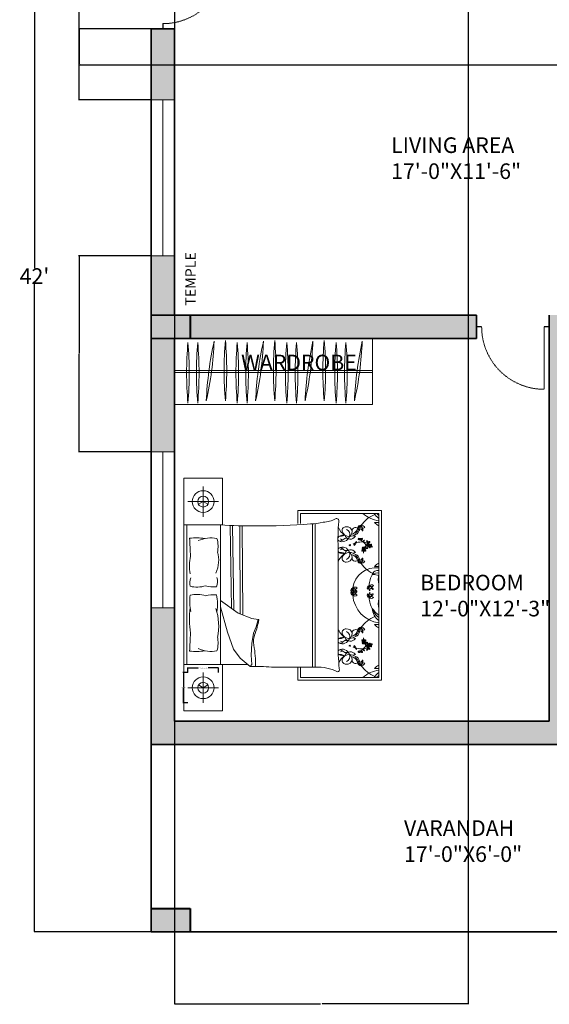
# Model space of a CAD drawing. Units: inches. Extents: x -10 to 455, y -513 to 57.
# Tile 1 of 4: x -10 to 193, y -513 to -134. Entities that reach past the tile are written whole.
import ezdxf

# ---------------------------------------------------------------- set-up
doc = ezdxf.new("R2010")
doc.units = ezdxf.units.IN
doc.header["$MEASUREMENT"] = 0
doc.linetypes.add('DASHED2', pattern=[0.375, 0.25, -0.125])
for name, color, linetype, lineweight in [('A-ANNO-DIMS', 2, 'Continuous', 18), ('A-ANNO-TEXT', 7, 'Continuous', 18), ('A-AREA-IDEN', 7, 'Continuous', 18), ('A-COLS', 7, 'Continuous', 40), ('A-COLS-PATT', 1, 'Continuous', 13), ('A-DOOR', 40, 'DASHED2', 18), ('A-DOOR-FRAM', 7, 'Continuous', 25), ('A-FLOR-CASE', 8, 'Continuous', 18), ('A-FURN', 8, 'Continuous', 13), ('A-GLAZ', 222, 'Continuous', 18), ('A-WALL', 7, 'Continuous', 35), ('A-WALL-PATT', 152, 'Continuous', 13)]:
    doc.layers.add(name, color=color, linetype=linetype, lineweight=lineweight)
doc.styles.get("Standard").update_dxf_attribs({"font": 'arial.ttf'})
doc.dimstyles.get("Standard").update_dxf_attribs({"dimtxt": 0.18, "dimasz": 0.18, "dimexe": 0.18, "dimexo": 0.0625, "dimgap": 0.09, "dimtad": 0, "dimtih": 1, "dimtoh": 1, "dimdec": 0, "dimzin": 0, "dimdsep": 46, "dimlunit": 3, "dimtxsty": 'Standard', "dimcen": 0.09, "dimadec": 0, "dimazin": 0, "dimtfac": 1, "dimtdec": 0, "dimtofl": 0, "dimtmove": 0, "dimatfit": 3, "dimfxl": 1, "dimtolj": 1, "dimtzin": 0, "dimarcsym": 0})

# ---------------------------------------------------------------- blocks, each defined once
blk = doc.blocks.new('*D2')
at = {"layer": 'A-ANNO-DIMS', "color": 0, "lineweight": -2, "transparency": 16777216}
for p, q in [((40.18, 19.15), (-4.74, 19.15)), ((-4.56, 18.97), (-4.56, -229.75)), ((-4.56, -484.67), (-4.56, -235.95)), ((40.18, -484.85), (-4.74, -484.85))]:
    blk.add_line(p, q, dxfattribs=at)
at = {"layer": 'A-ANNO-DIMS', "color": 0, "transparency": 16777216}
for points in [[(-4.59, 18.97), (-4.53, 18.97), (-4.56, 19.15)], [(-4.59, -484.67), (-4.53, -484.67), (-4.56, -484.85)]]:
    blk.add_solid(points, dxfattribs=at)
at = {"layer": 'Defpoints', "color": 0, "transparency": 16777216}
for p in [(40.25, 19.15), (-4.56, -484.85), (40.25, -484.85)]:
    blk.add_point(p, dxfattribs=at)
at = {"layer": 'A-ANNO-DIMS', "color": 0, "transparency": 16777216, "insert": (-4.56, -232.85), "char_height": 6, "attachment_point": 5}
blk.add_mtext("\\A1;42'", dxfattribs=at)
blk = doc.blocks.new('WIN-60IN')
for p, q in [((0, 9), (60, 9)), ((0, 0), (0, 9)), ((60, 9), (60, 0)), ((0, 4.5), (60, 4.5)), ((60, 0), (0, 0))]:
    blk.add_line(p, q)
blk = doc.blocks.new('DOOR-SINGLE-24IN')
for p, q in [((0, 28), (0, 26)), ((0, 26), (24, 26)), ((0, 0), (0, 2))]:
    blk.add_line(p, q)
blk.add_arc((0, 26), 24, 270, 0)
blk = doc.blocks.new('LAMP-BEDSIDE-SMALL')
for p, q in [((5.84, 0), (5.84, 11.68)), ((11.68, 5.84), (0, 5.84))]:
    blk.add_line(p, q)
for points in [[(5.84, 5.84), (4.03, 4.8)], [(5.84, 5.84), (7.65, 4.8)]]:
    blk.add_lwpolyline(points)
for radius in [4.17, 2.09]:
    blk.add_circle((5.84, 5.84), radius)
blk = doc.blocks.new('*D28')
at = {"layer": 'A-ANNO-DIMS', "color": 0, "lineweight": -2, "transparency": 16777216}
for p, q in [((54.41, -385.12), (54.41, -383.25)), ((54.59, -383.43), (58.38, -383.43)), ((65.92, -383.43), (62.13, -383.43)), ((66.1, -385.12), (66.1, -383.25))]:
    blk.add_line(p, q, dxfattribs=at)
at = {"layer": 'A-ANNO-DIMS', "color": 0, "transparency": 16777216}
for points in [[(54.59, -383.4), (54.59, -383.46), (54.41, -383.43)], [(65.92, -383.4), (65.92, -383.46), (66.1, -383.43)]]:
    blk.add_solid(points, dxfattribs=at)
at = {"layer": 'Defpoints', "color": 0, "transparency": 16777216}
for p in [(54.41, -383.43), (54.41, -385.18), (66.1, -385.18)]:
    blk.add_point(p, dxfattribs=at)
at = {"layer": 'A-ANNO-DIMS', "color": 0, "transparency": 16777216, "insert": (60.25, -383.43), "char_height": 0.18, "attachment_point": 5}
blk.add_mtext('\\A1;BEDSIDE LAMP 0\'-11 1/2" TYP.', dxfattribs=at)
blk = doc.blocks.new('*D29')
at = {"layer": 'A-ANNO-DIMS', "color": 0, "lineweight": -2, "transparency": 16777216}
for p, q in [((54.35, -385.18), (52.48, -385.18)), ((52.66, -385.36), (52.66, -390.84)), ((52.66, -396.68), (52.66, -391.2)), ((54.35, -396.86), (52.48, -396.86))]:
    blk.add_line(p, q, dxfattribs=at)
at = {"layer": 'A-ANNO-DIMS', "color": 0, "transparency": 16777216}
for points in [[(52.63, -385.36), (52.69, -385.36), (52.66, -385.18)], [(52.63, -396.68), (52.69, -396.68), (52.66, -396.86)]]:
    blk.add_solid(points, dxfattribs=at)
at = {"layer": 'Defpoints', "color": 0, "transparency": 16777216}
for p in [(54.41, -385.18), (52.66, -396.86), (54.41, -396.86)]:
    blk.add_point(p, dxfattribs=at)
at = {"layer": 'A-ANNO-DIMS', "color": 0, "transparency": 16777216, "insert": (52.66, -391.02), "char_height": 0.18, "attachment_point": 5}
blk.add_mtext('\\A1;0\'-11 1/2" TYP.', dxfattribs=at)
blk = doc.blocks.new('*D35')
at = {"layer": 'A-ANNO-DIMS', "color": 0, "lineweight": -2, "transparency": 16777216}
for p, q in [((40.18, -137.85), (12.42, -137.85)), ((12.6, -138.03), (12.6, -151.3)), ((12.6, -164.93), (12.6, -151.67)), ((40.18, -165.11), (12.42, -165.11))]:
    blk.add_line(p, q, dxfattribs=at)
at = {"layer": 'A-ANNO-DIMS', "color": 0, "transparency": 16777216}
for points in [[(12.57, -138.03), (12.63, -138.03), (12.6, -137.85)], [(12.57, -164.93), (12.63, -164.93), (12.6, -165.11)]]:
    blk.add_solid(points, dxfattribs=at)
at = {"layer": 'Defpoints', "color": 0, "transparency": 16777216}
for p in [(40.25, -137.85), (12.6, -165.11), (40.25, -165.11)]:
    blk.add_point(p, dxfattribs=at)
at = {"layer": 'A-ANNO-DIMS', "color": 0, "transparency": 16777216, "insert": (12.6, -151.48), "char_height": 0.18, "attachment_point": 5}
blk.add_mtext('\\A1;2\'-3 1/2"', dxfattribs=at)
blk = doc.blocks.new('*D36')
at = {"layer": 'A-ANNO-DIMS', "color": 0, "lineweight": -2, "transparency": 16777216}
for p, q in [((40.18, -225.11), (12.42, -225.11)), ((12.6, -225.29), (12.6, -262.55)), ((12.6, -300.17), (12.6, -262.91)), ((40.18, -300.35), (12.42, -300.35))]:
    blk.add_line(p, q, dxfattribs=at)
at = {"layer": 'A-ANNO-DIMS', "color": 0, "transparency": 16777216}
for points in [[(12.57, -225.29), (12.63, -225.29), (12.6, -225.11)], [(12.57, -300.17), (12.63, -300.17), (12.6, -300.35)]]:
    blk.add_solid(points, dxfattribs=at)
at = {"layer": 'Defpoints', "color": 0, "transparency": 16777216}
for p in [(40.25, -225.11), (12.6, -300.35), (40.25, -300.35)]:
    blk.add_point(p, dxfattribs=at)
at = {"layer": 'A-ANNO-DIMS', "color": 0, "transparency": 16777216, "insert": (12.6, -262.73), "char_height": 0.18, "attachment_point": 5}
blk.add_mtext('\\A1;6\'-3"', dxfattribs=at)
blk = doc.blocks.new('*D43')
at = {"layer": 'A-ANNO-DIMS', "color": 0, "lineweight": -2, "transparency": 16777216}
for p, q in [((253.18, -109.85), (12.42, -109.85)), ((12.6, -110.03), (12.6, -130.67)), ((12.6, -151.67), (12.6, -131.03)), ((253.18, -151.85), (12.42, -151.85))]:
    blk.add_line(p, q, dxfattribs=at)
at = {"layer": 'A-ANNO-DIMS', "color": 0, "transparency": 16777216}
for points in [[(12.57, -110.03), (12.63, -110.03), (12.6, -109.85)], [(12.57, -151.67), (12.63, -151.67), (12.6, -151.85)]]:
    blk.add_solid(points, dxfattribs=at)
at = {"layer": 'Defpoints', "color": 0, "transparency": 16777216}
for p in [(253.25, -109.85), (12.6, -151.85), (253.25, -151.85)]:
    blk.add_point(p, dxfattribs=at)
at = {"layer": 'A-ANNO-DIMS', "color": 0, "transparency": 16777216, "insert": (12.6, -130.85), "char_height": 0.18, "attachment_point": 5}
blk.add_mtext('\\A1;3\'-6"', dxfattribs=at)
blk = doc.blocks.new('*D44')
at = {"layer": 'A-ANNO-DIMS', "color": 0, "lineweight": -2, "transparency": 16777216}
for p, q in [((49.25, 10.09), (49.25, -512.68)), ((162.09, 10.09), (162.09, -512.68)), ((49.43, -512.5), (105.34, -512.5)), ((161.91, -512.5), (106, -512.5))]:
    blk.add_line(p, q, dxfattribs=at)
at = {"layer": 'A-ANNO-DIMS', "color": 0, "transparency": 16777216}
for points in [[(49.43, -512.47), (49.43, -512.53), (49.25, -512.5)], [(161.91, -512.47), (161.91, -512.53), (162.09, -512.5)]]:
    blk.add_solid(points, dxfattribs=at)
at = {"layer": 'Defpoints', "color": 0, "transparency": 16777216}
for p in [(49.25, 10.15), (162.09, 10.15), (162.09, -512.5)]:
    blk.add_point(p, dxfattribs=at)
at = {"layer": 'A-ANNO-DIMS', "color": 0, "transparency": 16777216, "insert": (105.67, -512.5), "char_height": 0.18, "attachment_point": 5}
blk.add_mtext('\\A1;9\'-5"', dxfattribs=at)

msp = doc.modelspace()

# ---------------------------------------------------------------- hatches: boundary and pattern name
at = {"layer": 'A-COLS-PATT'}
h = msp.add_hatch(color=256, dxfattribs=at)
h.dxf.hatch_style = 1
h.paths.add_polyline_path([(55.25, 19.15), (40.25, 19.15), (40.25, 10.15), (55.25, 10.15)])
h.paths.add_polyline_path([(262.25, 19.15), (253.25, 19.15), (253.25, 4.15), (262.25, 4.15)])
h.paths.add_polyline_path([(427.25, 19.15), (418.25, 19.15), (418.25, 4.15), (427.25, 4.15)])
h.paths.add_polyline_path([(427.25, -247.85), (418.25, -247.85), (418.25, -262.85), (427.25, -262.85)])
h.paths.add_polyline_path([(268.25, -247.85), (253.25, -247.85), (253.25, -256.85), (268.25, -256.85)])
h.paths.add_polyline_path([(55.25, -247.85), (40.25, -247.85), (40.25, -256.85), (55.25, -256.85)])
h.paths.add_polyline_path([(55.25, -475.85), (49.25, -475.85), (40.25, -475.85), (40.25, -484.85), (55.25, -484.85)])
h.paths.add_polyline_path([(268.25, -475.85), (253.25, -475.85), (253.25, -484.85), (268.25, -484.85)])
h.paths.add_polyline_path([(427.25, -469.85), (418.25, -469.85), (418.25, -484.85), (427.25, -484.85)])
h.paths.add_polyline_path([(55.25, -100.85), (40.25, -100.85), (40.25, -109.85), (55.25, -109.85)])
at = {"layer": 'A-WALL-PATT'}
h = msp.add_hatch(color=256, dxfattribs=at)
h.dxf.hatch_style = 1
h.paths.add_polyline_path([(418.25, -151.85), (268.25, -151.85), (268.25, -160.85), (418.25, -160.85)])
h.paths.add_polyline_path([(165.25, -100.85), (55.25, -100.85), (55.25, -109.85), (165.25, -109.85), (165.25, -105.35)])
h.paths.add_polyline_path([(49.25, -75.35), (40.25, -75.35), (40.25, -100.85), (49.25, -100.85)])
h.paths.add_polyline_path([(49.25, 10.15), (40.25, 10.15), (40.25, -15.35), (49.25, -15.35)])
h.paths.add_polyline_path([(86.75, 19.15), (55.25, 19.15), (55.25, 10.15), (86.75, 10.15)])
h.paths.add_polyline_path([(213.5, 19.15), (146.75, 19.15), (146.75, 10.15), (193.25, 10.15), (193.25, -28.04), (197.75, -28.04), (197.75, 10.15), (213.5, 10.15)])
h.paths.add_polyline_path([(262.25, 4.15), (253.25, 4.15), (253.25, -69.35), (197.75, -69.35), (197.75, -60), (193.25, -60), (193.25, -109.85), (197.75, -109.85), (197.75, -73.85), (253.25, -73.85), (253.25, -109.85), (262.25, -109.85)])
h.paths.add_polyline_path([(310.25, 19.15), (262.25, 19.15), (262.25, 10.15), (310.25, 10.15)])
h.paths.add_polyline_path([(253.25, 19.15), (237.5, 19.15), (237.5, 10.15), (253.25, 10.15)])
h.paths.add_polyline_path([(418.25, 19.15), (370.25, 19.15), (370.25, 10.15), (418.25, 10.15)])
h.paths.add_polyline_path([(427.25, 4.15), (418.25, 4.15), (418.25, -42.17), (427.25, -42.17)])
h.paths.add_polyline_path([(427.25, -102.17), (418.25, -102.17), (418.25, -145.85), (427.25, -145.85)])
h.paths.add_polyline_path([(427.25, -160.85), (418.25, -160.85), (418.25, -247.85), (427.25, -247.85)])
h.paths.add_polyline_path([(418.25, -247.85), (365.75, -247.85), (365.75, -256.85), (418.25, -256.85)], flags=17)
h.paths.add_polyline_path([(297.25, -247.85), (268.25, -247.85), (268.25, -256.85), (297.25, -256.85), (297.25, -252.35)], flags=17)
h.paths.add_polyline_path([(427.25, -299.44), (418.25, -299.44), (418.25, -319.85), (370.25, -319.85), (370.25, -284.85), (368, -284.85), (365.75, -284.85), (365.75, -319.85), (329.75, -319.85), (329.75, -247.85), (325.25, -247.85), (325.25, -319.85), (257.75, -319.85), (257.75, -256.85), (253.25, -256.85), (253.25, -324.35), (262.25, -324.35), (418.25, -324.35), (418.25, -363.39), (427.25, -363.39)])
h.paths.add_polyline_path([(262.25, -352.35), (257.75, -352.35), (253.25, -352.35), (253.25, -447.85), (257.75, -447.85), (262.25, -447.85)])
h.paths.add_polyline_path([(305.75, -475.85), (268.25, -475.85), (268.25, -484.85), (305.75, -484.85)])
h.paths.add_polyline_path([(418.25, -475.85), (365.75, -475.85), (365.75, -484.85), (418.25, -484.85)])
h.paths.add_polyline_path([(427.25, -423.39), (418.25, -423.39), (418.25, -469.85), (427.25, -469.85)])
h.paths.add_polyline_path([(202.25, -247.85), (193.25, -247.85), (193.25, -403.85), (49.25, -403.85), (49.25, -360.35), (40.25, -360.35), (40.25, -412.85), (202.25, -412.85)])
h.paths.add_polyline_path([(165.25, -247.85), (55.25, -247.85), (55.25, -256.85), (165.25, -256.85), (165.25, -252.35)], flags=17)
h.paths.add_polyline_path([(49.25, -225.11), (40.25, -225.11), (40.25, -247.85), (49.25, -247.85)])
h.paths.add_polyline_path([(49.25, -256.85), (40.25, -256.85), (40.25, -300.35), (49.25, -300.35)], flags=17)
h.paths.add_polyline_path([(49.25, -137.85), (44.75, -137.85), (40.25, -137.85), (40.25, -165.11), (49.25, -165.11)])

# ---------------------------------------------------------------- linework, layer by layer
at = {"layer": 'A-COLS'}
for p, q in [((55.25, -247.85), (55.25, -256.85)), ((40.25, -475.85), (49.25, -475.85)), ((49.25, -475.85), (55.25, -475.85)), ((55.25, -475.85), (55.25, -484.85))]:
    msp.add_line(p, q, dxfattribs=at)
at = {"layer": 'A-DOOR-FRAM'}
for p, q in [((44.75, -135.85), (44.75, -137.85)), ((167.25, -252.35), (165.25, -252.35)), ((193.25, -252.35), (191.25, -252.35))]:
    msp.add_line(p, q, dxfattribs=at)
at = {"layer": 'A-FLOR-CASE'}
for p, q in [((125.31, -256.85), (49.25, -256.85)), ((49.25, -256.85), (49.25, -282.2)), ((125.31, -256.85), (125.31, -282.2)), ((125.31, -269.1), (49.25, -269.1)), ((125.31, -269.95), (49.25, -269.95)), ((125.31, -282.2), (49.25, -282.2))]:
    msp.add_line(p, q, dxfattribs=at)
for centre, start, end in [((187.3, -270.03), 175.0028, 184.9972), ((-78.5, -270.03), 355.0028, 4.9972), ((191.06, -270.03), 175.0028, 184.9972), ((-74.74, -270.03), 355.0028, 4.9972), ((-68.8, -251.99), 347.508, 357.5023), ((194.73, -286.66), 167.508, 177.5023), ((201.69, -269.22), 175.0028, 184.9972), ((-64.11, -269.22), 355.0028, 4.9972), ((206.26, -270.03), 175.0028, 184.9972), ((-59.54, -270.03), 355.0028, 4.9972), ((210.01, -270.03), 175.0028, 184.9972), ((-55.79, -270.03), 355.0028, 4.9972), ((-49.85, -251.99), 347.508, 357.5023), ((213.68, -286.66), 167.508, 177.5023), ((220.64, -269.22), 175.0028, 184.9972), ((-45.16, -269.22), 355.0028, 4.9972), ((225.28, -270.03), 175.0028, 184.9972), ((-40.52, -270.03), 355.0028, 4.9972), ((229.03, -270.03), 175.0028, 184.9972), ((-36.77, -270.03), 355.0028, 4.9972), ((232.7, -286.66), 167.508, 177.5023), ((-30.83, -251.99), 347.508, 357.5023), ((239.66, -269.22), 175.0028, 184.9972), ((-26.14, -269.22), 355.0028, 4.9972), ((244.23, -270.03), 175.0028, 184.9972), ((-21.57, -270.03), 355.0028, 4.9972), ((247.98, -270.03), 175.0028, 184.9972), ((-17.82, -270.03), 355.0028, 4.9972), ((251.65, -286.66), 167.508, 177.5023), ((-11.88, -251.99), 347.508, 357.5023)]:
    msp.add_arc(centre, 133.41, start, end, dxfattribs=at)
at = {"layer": 'A-FURN'}
for p, q in [((52.81, -399.96), (52.81, -310.56)), ((96.63, -327.95), (96.63, -322.99)), ((96.63, -322.99), (128.83, -322.99)), ((97.66, -324.02), (97.66, -327.96)), ((127.79, -324.02), (97.66, -324.02)), ((127.79, -387.12), (127.79, -324.02)), ((128.83, -322.99), (128.83, -388.16)), ((53.95, -328.44), (53.95, -382.08)), ((66.93, -382.08), (66.93, -328.44)), ((70.65, -328.68), (71.09, -360.51)), ((71.56, -328.72), (72.02, -361.18)), ((74.38, -328.76), (74.51, -362.71)), ((75.3, -328.76), (75.44, -363.06)), ((102.2, -328.04), (102.2, -383.11)), ((103.32, -327.95), (103.32, -383.11)), ((118.73, -332.83), (117.72, -332.64)), ((112.1, -337.11), (112.1, -373.41)), ((118.73, -339.08), (117.72, -339.28)), ((66.93, -357.52), (73.75, -362.42)), ((69.59, -369.66), (66.93, -359.92)), ((73.75, -362.42), (79, -364.41)), ((79, -364.41), (81.35, -364.78)), ((81.35, -364.78), (80.63, -367.67)), ((71.94, -376.18), (69.59, -369.66)), ((79.54, -370.03), (79, -374.01)), ((80.63, -367.67), (79.54, -370.03)), ((79, -374.01), (78.64, -378.54)), ((118.73, -372.07), (117.72, -371.87)), ((74.47, -379.62), (71.94, -376.18)), ((118.73, -378.32), (117.72, -378.51)), ((52.81, -382.08), (77.34, -382.08)), ((78.27, -382.88), (74.47, -379.62)), ((78.64, -378.54), (79, -382.16)), ((79, -382.16), (78.27, -382.88)), ((96.63, -388.16), (96.63, -383.1)), ((97.66, -383.11), (97.66, -387.12)), ((128.83, -388.16), (96.63, -388.16)), ((97.66, -387.12), (127.79, -387.12))]:
    msp.add_line(p, q, dxfattribs=at)
for points in [[(52.81, -328.44), (67.7, -328.44), (67.7, -310.56), (52.81, -310.56)], [(67.7, -382.08), (67.7, -399.96), (52.81, -399.96)]]:
    msp.add_lwpolyline(points, dxfattribs=at)
for points in [[(101.5, -328.06, 0.056112), (106.42, -327.41, 0.095341), (111.15, -326.16)], [(55.03, -333.58, -0.074897), (60.87, -333.69, 0.472817)], [(61.2, -351.86, -0.14099), (55.24, -352.04, -0.235245)], [(61.2, -355.68, 0.14099), (55.24, -355.5, 0.235245)], [(55.03, -376.95, 0.074897), (60.87, -376.84, -0.472817)], [(86.46, -383.07, 0.001242), (103.42, -383.11, -0.127202), (111.88, -384.9)]]:
    msp.add_lwpolyline(points, format="xyb", dxfattribs=at)
for centre in [(124.37, -336.51), (121.97, -338), (121.97, -373.15), (124.37, -374.64)]:
    msp.add_circle(centre, 0.228, dxfattribs=at)
for centre, radius, start, end in [((130.52, -335.3), 11.67, 111.4092, 145.6135), ((129.37, -315.33), 11.67, 228.1144, 262.255), ((130.93, -321.19), 5.69, 209.8884, 236.5383), ((131.99, -319.14), 7.09, 223.5186, 233.6964), ((77.86, -168.19), 160.63, 266.1, 270.9282), ((83.7, -119.29), 209.53, 269.1145, 274.8735), ((111.61, -326.83), 0.815, 336.5219, 123.8264), ((199.04, -334.38), 86.99, 175.2402, 181.8035), ((115.15, -330.66), 1.51, 88.9462, 185.5144), ((115.36, -331.28), 2.14, 7.1143, 95.0551), ((120.66, -329.65), 0.968, 76.272, 177.0484), ((119.19, -327.67), 1.99, 284.7031, 328.6173), ((121.97, -330.21), 1.85, 125.7657, 194.5347), ((112.92, -326.94), 8.17, 332.8176, 347.4827), ((121.16, -329.98), 1.29, 20.9613, 102.2885), ((121.86, -328.68), 0.975, 181.7131, 301.5367), ((118.67, -330.65), 2.95, 2.0648, 41.1598), ((120.44, -329.56), 0.955, 316.2238, 62.3173), ((129.61, -324.38), 4.75, 221.0454, 247.4453), ((127.06, -311.37), 16.15, 266.3481, 272.5919), ((113.09, -333.79), 1.08, 127.675, 162.5814), ((112.76, -329.2), 3.7, 259.249, 301.1782), ((118.39, -326.72), 6.77, 203.6453, 236.3329), ((114.37, -335.79), 3.45, 85.2696, 124.215), ((116.26, -330.2), 2.69, 193.079, 274.7067), ((116.8, -331.73), 2.22, 196.8663, 330.0915), ((114.55, -332.12), 2.07, 338.5779, 68.4181), ((114.37, -335.79), 3.45, 53.6555, 57.2989), ((114.89, -330.91), 2.6, 305.9599, 357.6409), ((116.19, -328.09), 4.8, 273.4924, 303.7117), ((115.85, -328.13), 4.22, 288.2955, 328.7386), ((118.8, -330.79), 1.34, 19.1312, 189.736), ((118.4, -330.47), 1.68, 285.6955, 4.031), ((120.63, -332.27), 1.78, 128.4175, 173.8338), ((120.26, -330.51), 0.822, 126.7319, 206.0245), ((120.99, -330.12), 0.0761, 20.2667, 316.2271), ((121.4, -330.54), 0.0704, 52.0591, 168.5166), ((121.47, -330.55), 0.145, 168.5166, 2.0648), ((-795.72, -382.85), 852.18, 2.85022, 3.31479), ((63.22, -344.97), 11.52, 78.2417, 114.8684), ((53.99, -336.77), 11.98, 348.9631, 14.8961), ((113.09, -333.79), 1.08, 196.6343, 225.5483), ((113.72, -332.07), 2.85, 240.8249, 340.7178), ((112.87, -333.33), 1.34, 246.1646, 318.4347), ((114.24, -331.64), 2.57, 240.0851, 262.564), ((115.25, -335.44), 1.83, 74.8529, 138.4347), ((115.87, -333.13), 0.555, 254.8529, 12.6959), ((116.61, -336.19), 0.28, 169.5864, 349.5616), ((116.71, -336.21), 0.172, 349.5616, 167.2949), ((121.21, -342.41), 7.4, 110.1059, 116.9968), ((117.38, -335.22), 1.41, 308.4388, 328.836), ((118.73, -336.31), 0.469, 129.5056, 182.6421), ((117.13, -334.07), 2.52, 296.5064, 305.3102), ((117.11, -335.37), 1.44, 336.3901, 344.4871), ((118.68, -335.74), 0.182, 83.9457, 185.6216), ((117.95, -335.57), 0.749, 328.836, 0.8141), ((118.34, -335.79), 0.429, 306.5232, 32.4668), ((118.85, -335.45), 0.182, 112.5583, 214.2343), ((118.73, -335.13), 0.429, 265.7131, 351.6568), ((118.35, -334.89), 0.749, 297.3659, 329.344), ((117.79, -334.25), 1.44, 313.6929, 321.7899), ((119.38, -335.23), 0.469, 115.5379, 168.6744), ((117.78, -334.55), 1.41, 329.344, 349.7412), ((121.21, -342.41), 7.4, 86.1723, 106.4158), ((116.65, -334.88), 2.52, 352.8698, 1.6736), ((119.99, -333.97), 0.176, 125.0752, 284.7644), ((120.26, -333.9), 0.38, 127.3642, 168.4363), ((119.97, -333.59), 0.547, 277.4968, 341.2737), ((120.4, -333.85), 0.217, 88.1325, 178.8919), ((120.84, -334.08), 0.471, 136.3462, 189.6513), ((120.57, -334.13), 0.196, 189.6513, 312.3208), ((120.62, -333.58), 0.228, 183.2768, 356.7232), ((121.33, -333.99), 0.745, 164.2829, 186.9148), ((120.45, -334), 0.373, 312.3208, 40.2111), ((121.24, -333.58), 0.529, 201.6382, 274.947), ((120.54, -334.3), 0.691, 42.3896, 66.5724), ((127.51, -328.83), 8.49, 217.9541, 226.8459), ((121.04, -333.89), 0.376, 10.9597, 52.2379), ((121.27, -333.93), 0.175, 274.947, 37.5263), ((121.86, -334.92), 0.182, 112.5583, 214.2343), ((121.74, -334.59), 0.429, 265.7131, 351.6568), ((121.36, -334.36), 0.749, 297.3659, 329.344), ((121.4, -338.72), 3.71, 60.7959, 85.244), ((113.49, -344.07), 12.21, 37.8256, 47.7588), ((120.79, -333.71), 1.44, 313.6929, 321.7899), ((122.38, -334.69), 0.469, 115.5379, 168.6744), ((120.79, -334.02), 1.41, 329.344, 349.7412), ((119.66, -334.34), 2.52, 352.8698, 1.6736), ((126.33, -339.1), 4.45, 130.182, 149.456), ((123.21, -334.85), 0.254, 33.0979, 123.1364), ((117.61, -338.44), 6.65, 31.1156, 34.8118), ((122.84, -335.29), 0.688, 2.3172, 70.5201), ((123.88, -336.57), 0.734, 139.3812, 199.9959), ((122.51, -336.03), 1.04, 310.9365, 22.7695), ((122.98, -336.09), 0.754, 285.6484, 332.2957), ((123.41, -335.46), 0.199, 135.7354, 318.1297), ((123.08, -335.14), 0.263, 315.7354, 31.1156), ((122.86, -335.69), 0.611, 319.3812, 5.5456), ((123.56, -335.46), 0.199, 68.2452, 250.6395), ((123.1, -335.21), 0.593, 352.6008, 57.1845), ((125.22, -339.19), 3.97, 111.7087, 116.2181), ((121.4, -338.72), 3.71, 47.5083, 55.9967), ((123.66, -335.08), 0.593, 252.8042, 349.6943), ((123.1, -336.14), 0.631, 331.1838, 51.6792), ((123.73, -335.03), 0.263, 248.2452, 323.6254), ((124.02, -336.82), 0.38, 93.635, 168.4363), ((123.49, -334.87), 0.688, 291.7087, 3.0299), ((123.97, -336.22), 0.223, 138.2946, 276.2474), ((123.72, -336.52), 0.547, 277.4968, 341.2737), ((124.05, -336.26), 0.31, 358.5719, 143.8954), ((118.58, -331.24), 6.65, 323.6254, 327.3216), ((124.15, -336.77), 0.217, 88.1325, 178.8919), ((124.23, -336.01), 0.313, 208.8493, 269.9355), ((123.97, -336.09), 0.358, 274.2123, 318.1587), ((124.59, -337.01), 0.471, 136.3462, 189.6513), ((124.04, -335.04), 0.254, 325.6077, 55.6462), ((125.08, -336.92), 0.745, 164.2829, 186.9148), ((125.06, -336.45), 0.718, 121.9501, 165.2442), ((124.2, -336.92), 0.373, 312.3208, 40.2111), ((124.99, -336.5), 0.529, 201.6382, 274.947), ((124.56, -336.17), 0.151, 262.868, 7.094), ((124.29, -337.22), 0.691, 42.3896, 66.5724), ((124.54, -336.05), 0.449, 278.5614, 22.5914), ((124.79, -336.82), 0.376, 10.9597, 118.7804), ((124.8, -336.03), 0.226, 44.3732, 121.9501), ((70.68, -344.19), 15.72, 166.3427, 191.1841), ((54.87, -341.94), 11.38, 333.8761, 16.1746), ((113.09, -338.13), 1.08, 134.4517, 156.7144), ((113.09, -338.13), 1.08, 203.2856, 232.325), ((112.76, -342.71), 3.7, 58.8218, 100.2867), ((118.39, -345.19), 6.77, 123.6671, 158.5059), ((113.72, -339.84), 2.85, 19.2822, 119.1751), ((112.87, -338.58), 1.34, 41.5653, 113.8354), ((114.37, -336.13), 3.45, 235.785, 274.7304), ((114.24, -340.27), 2.57, 97.436, 119.9149), ((116.26, -341.72), 2.69, 85.2933, 166.921), ((115.25, -336.48), 1.83, 221.5653, 285.1471), ((116.8, -340.19), 2.22, 29.9085, 163.1337), ((114.55, -339.79), 2.07, 291.5819, 21.4221), ((115.87, -338.78), 0.555, 347.3041, 105.1471), ((114.37, -336.13), 3.45, 302.7011, 306.3445), ((114.89, -341.01), 2.6, 2.3591, 54.0401), ((116.19, -343.83), 4.8, 56.2883, 86.5076), ((115.85, -343.79), 4.22, 31.2614, 71.7045), ((120.63, -339.64), 1.78, 186.1662, 231.5825), ((118.4, -341.45), 1.68, 355.969, 74.3045), ((121.35, -338.38), 0.176, 125.0752, 284.7644), ((121.62, -338.31), 0.38, 93.635, 168.4363), ((121.63, -336.26), 1.04, 253.6301, 325.4631), ((121.92, -337.7), 0.734, 82.0748, 142.6895), ((121.84, -336.69), 0.754, 228.342, 274.9894), ((121.57, -337.71), 0.223, 138.2946, 276.2474), ((121.32, -338.01), 0.547, 277.4968, 341.2737), ((121.65, -337.75), 0.31, 358.5719, 143.8954), ((121.75, -338.26), 0.217, 88.1325, 178.8919), ((121.83, -337.5), 0.313, 208.8493, 269.9355), ((121.57, -337.58), 0.358, 274.2123, 318.1587), ((122.19, -338.49), 0.471, 136.3462, 189.6513), ((121.92, -338.54), 0.196, 189.6513, 312.3208), ((126.33, -339.1), 4.45, 175.2415, 182.8929), ((121.86, -336.81), 0.631, 273.8774, 357.1501), ((122.68, -338.4), 0.745, 164.2829, 186.9148), ((122.66, -337.94), 0.718, 121.9501, 165.2442), ((122.11, -336.36), 0.611, 262.0748, 308.2393), ((121.8, -338.41), 0.373, 312.3208, 40.2111), ((122.59, -337.99), 0.529, 201.6382, 274.947), ((122.16, -337.66), 0.151, 262.868, 7.094), ((121.89, -338.71), 0.691, 42.3896, 66.5724), ((122.14, -337.53), 0.449, 278.5614, 22.5914), ((122.39, -338.31), 0.376, 10.9597, 118.7804), ((126.33, -339.1), 4.45, 156.1523, 156.9499), ((122.4, -337.52), 0.226, 44.3732, 121.9501), ((123.09, -336.99), 0.631, 181.4625, 249.4747), ((122.99, -336.49), 0.611, 215.1128, 261.2773), ((123.47, -336.52), 1.04, 197.889, 269.722), ((122.62, -338.34), 0.175, 274.947, 37.5263), ((123.15, -336.88), 0.754, 248.3627, 295.0101), ((122.78, -337.82), 0.734, 20.6625, 81.2773), ((123.75, -336.89), 0.176, 125.0752, 284.7644), ((124.32, -337.05), 0.196, 189.6513, 312.3208), ((125.02, -336.85), 0.175, 274.947, 37.5263), ((115.15, -341.25), 1.51, 174.4856, 271.0538), ((115.36, -340.63), 2.14, 264.9449, 352.8857), ((118.8, -341.13), 1.34, 170.264, 340.8688), ((120.26, -341.4), 0.822, 153.9755, 233.2681), ((120.66, -342.26), 0.968, 182.9516, 283.728), ((119.19, -344.24), 1.99, 31.3827, 75.2969), ((121.97, -341.7), 1.85, 165.4653, 234.2343), ((112.92, -344.97), 8.17, 12.5173, 27.1824), ((118.67, -341.26), 2.95, 318.8402, 357.9352), ((120.44, -342.36), 0.955, 297.6827, 43.7762), ((121.86, -343.23), 0.975, 58.4633, 178.2869), ((121.16, -341.94), 1.29, 257.7115, 339.0387), ((130.52, -336.61), 11.67, 214.3865, 248.5908), ((121.04, -341.78), 0.126, 43.7762, 339.7183), ((121.47, -341.36), 0.145, 357.9352, 191.4834), ((121.4, -341.38), 0.0704, 191.4834, 307.9409), ((129.61, -347.54), 4.75, 112.5547, 138.9546), ((126.67, -353.98), 9.03, 82.8636, 171.8197), ((135.62, -352.71), 11.67, 152.5854, 175.5377), ((127.3, -348.02), 2.1, 76.3898, 169.0739), ((127.01, -349.59), 2.65, 72.8609, 131.9049), ((125.85, -352.81), 5.23, 68.117, 96.6195), ((127.06, -360.54), 16.15, 87.4081, 93.6519), ((133.93, -349.44), 6.42, 162.9798, 196.4569), ((59.49, -350.82), 4.42, 153.3437, 196.1026), ((64.19, -341.33), 10.95, 254.1707, 275.9871), ((61.03, -350.22), 4.74, 335.0183, 18.5407), ((124.25, -352.73), 0.968, 106.1963, 206.9726), ((121.99, -351.75), 1.99, 314.6273, 358.5415), ((125.66, -352.56), 1.85, 155.6899, 224.4589), ((124.85, -352.76), 1.29, 50.8855, 132.2127), ((124.81, -351.29), 0.975, 211.6373, 331.4609), ((123.02, -354.59), 2.95, 31.989, 71.0841), ((116.19, -354.24), 8.17, 2.7418, 17.407), ((124.02, -352.75), 0.955, 346.148, 92.2415), ((137.24, -351.99), 9.49, 174.3643, 175.6213), ((143.74, -356.99), 16.96, 160.0972, 160.2783), ((71, -357.85), 15.93, 171.5249, 193.96), ((64.19, -366.22), 10.95, 84.0129, 105.8293), ((50.01, -359.04), 15.76, 349.8617, 13.6238), ((118, -353.62), 0.968, 106.1963, 206.9726), ((118, -354.55), 0.968, 153.0274, 253.8037), ((115.74, -352.64), 1.99, 314.6273, 358.5415), ((115.74, -355.53), 1.99, 1.4585, 45.3727), ((119.41, -353.45), 1.85, 155.6899, 224.4589), ((119.41, -354.72), 1.85, 135.5411, 204.3101), ((118.6, -353.65), 1.29, 50.8855, 132.2127), ((118.56, -352.18), 0.975, 211.6373, 331.4609), ((117.77, -353.65), 0.955, 346.148, 92.2415), ((116.77, -355.49), 2.95, 31.989, 71.0841), ((109.94, -355.14), 8.17, 2.7418, 17.407), ((109.94, -353.03), 8.17, 342.593, 357.2582), ((116.77, -352.68), 2.95, 288.9159, 328.011), ((117.77, -354.52), 0.955, 267.7585, 13.852), ((118.56, -355.99), 0.975, 28.5391, 148.3627), ((118.6, -354.52), 1.29, 227.7873, 309.1145), ((129.37, -354.57), 11.67, 184.4623, 262.255), ((118.57, -354.32), 0.126, 13.852, 309.9245), ((118.52, -353.86), 0.0761, 50.1909, 346.0209), ((119.08, -354.02), 0.0704, 81.9833, 198.4408), ((119.08, -354.15), 0.0704, 161.5592, 278.0167), ((119.15, -354), 0.145, 198.4408, 31.989), ((119.15, -354.17), 0.145, 328.011, 161.5592), ((124.25, -355.44), 0.968, 153.0274, 253.8037), ((121.99, -356.42), 1.99, 1.4585, 45.3727), ((125.66, -355.61), 1.85, 135.5411, 204.3101), ((116.19, -353.93), 8.17, 342.593, 357.2582), ((123.02, -353.58), 2.95, 288.9159, 328.011), ((124.02, -355.42), 0.955, 267.7585, 13.852), ((124.77, -352.96), 0.0761, 50.1909, 346.0209), ((124.82, -355.22), 0.126, 13.852, 309.9245), ((125.33, -353.13), 0.0704, 81.9833, 198.4408), ((125.33, -355.04), 0.0704, 161.5592, 278.0167), ((125.41, -353.11), 0.145, 198.4408, 31.989), ((125.41, -355.06), 0.145, 328.011, 161.5592), ((124.81, -356.88), 0.975, 28.5391, 148.3627), ((124.85, -355.41), 1.29, 227.7873, 309.1145), ((135.62, -355.46), 11.67, 184.4623, 207.4146), ((133.93, -358.73), 6.42, 163.5431, 197.0202), ((137.24, -356.18), 9.49, 184.3787, 185.6357), ((143.74, -351.18), 16.96, 199.7217, 199.9028), ((87.38, -364.7), 32.42, 172.2196, 189.497), ((45.47, -367.45), 20.78, 348.0397, 19.2615), ((130.93, -360.42), 5.69, 181.272, 236.5383), ((133.98, -354.65), 10.54, 214.0123, 234.053), ((131.99, -358.38), 7.09, 197.8504, 233.6964), ((47.57, -358.57), 34.67, 340.1194, 349.3383), ((81.42, -364.98), 0.216, 358.8623, 109.7536), ((130.52, -374.54), 11.67, 111.4092, 145.6135), ((127.06, -350.61), 16.15, 266.3481, 272.5919), ((129.61, -363.61), 4.75, 221.0454, 247.4453), ((-795.72, -327.67), 852.18, 356.68521, 357.14978), ((86.83, -373.29), 7.28, 156.2616, 191.3392), ((118.39, -365.95), 6.77, 201.4941, 236.3329), ((115.15, -369.9), 1.51, 88.9462, 185.5144), ((116.26, -369.43), 2.69, 193.079, 274.7067), ((115.36, -370.51), 2.14, 7.1143, 95.0551), ((114.55, -371.35), 2.07, 338.5779, 68.4181), ((114.89, -370.14), 2.6, 305.9599, 357.6409), ((115.85, -367.36), 4.22, 288.2955, 328.7386), ((118.8, -370.02), 1.34, 19.1312, 189.736), ((118.4, -369.7), 1.68, 285.6955, 4.031), ((120.63, -371.51), 1.78, 128.4175, 173.8338), ((120.26, -369.75), 0.822, 126.7319, 206.0245), ((120.66, -368.89), 0.968, 76.272, 177.0484), ((119.19, -366.91), 1.99, 284.7031, 328.6173), ((121.97, -369.44), 1.85, 125.7657, 194.5347), ((112.92, -366.18), 8.17, 332.8176, 347.4827), ((121.16, -369.21), 1.29, 20.9613, 102.2885), ((120.44, -368.79), 0.955, 316.2238, 62.3173), ((118.67, -369.89), 2.95, 2.0648, 41.1598), ((121.86, -367.92), 0.975, 181.7131, 301.5367), ((120.99, -369.35), 0.0761, 20.2667, 316.2271), ((121.4, -369.77), 0.0704, 52.0591, 168.5166), ((121.47, -369.79), 0.145, 168.5166, 2.0648), ((53.99, -373.76), 11.98, 345.1039, 11.0369), ((205.15, -374.48), 93.06, 179.3433, 185.6887), ((112.76, -368.44), 3.7, 259.7133, 301.1782), ((113.09, -373.02), 1.08, 127.675, 156.7144), ((113.09, -373.02), 1.08, 203.229, 225.5483), ((113.72, -371.3), 2.85, 240.8249, 340.7178), ((112.87, -372.57), 1.34, 246.1646, 318.4347), ((114.37, -375.02), 3.45, 85.2696, 124.215), ((114.24, -370.87), 2.57, 240.0851, 262.564), ((115.25, -374.67), 1.83, 74.8529, 138.4347), ((116.8, -370.96), 2.22, 196.8663, 330.0915), ((115.87, -372.37), 0.555, 254.8529, 12.6959), ((114.37, -375.02), 3.45, 53.6555, 57.2989), ((116.19, -367.32), 4.8, 273.4924, 303.7117), ((121.35, -372.77), 0.176, 75.2356, 234.9248), ((121.62, -372.84), 0.38, 191.5637, 266.365), ((121.84, -374.46), 0.754, 85.0106, 131.658), ((121.63, -374.89), 1.04, 34.5369, 106.3699), ((121.92, -373.45), 0.734, 217.3105, 277.9252), ((121.57, -373.44), 0.223, 83.7526, 221.7054), ((121.32, -373.14), 0.547, 18.7263, 82.5032), ((121.65, -373.4), 0.31, 216.1046, 1.4281), ((121.75, -372.89), 0.217, 181.1081, 271.8675), ((121.83, -373.65), 0.313, 90.0645, 151.1507), ((121.57, -373.57), 0.358, 41.8413, 85.7877), ((122.19, -372.65), 0.471, 170.3487, 223.6538), ((121.92, -372.61), 0.196, 47.6792, 170.3487), ((126.33, -372.05), 4.45, 177.1071, 184.7585), ((121.86, -374.34), 0.631, 2.8499, 86.1226), ((122.68, -372.74), 0.745, 173.0852, 195.7171), ((122.66, -373.21), 0.718, 194.7558, 238.0499), ((122.11, -374.79), 0.611, 51.7607, 97.9252), ((121.8, -372.74), 0.373, 319.7889, 47.6792), ((122.59, -373.16), 0.529, 85.053, 158.3618), ((122.16, -373.49), 0.151, 352.906, 97.132), ((121.89, -372.44), 0.691, 293.4276, 317.6104), ((122.39, -372.84), 0.376, 241.2196, 349.0403), ((122.14, -373.61), 0.449, 337.4086, 81.4386), ((126.33, -372.05), 4.45, 203.0501, 203.8477), ((122.4, -373.63), 0.226, 238.0499, 315.6268), ((123.09, -374.16), 0.631, 110.5253, 178.5375), ((123.47, -374.62), 1.04, 90.278, 162.111), ((122.99, -374.66), 0.611, 98.7227, 144.8872), ((126.33, -372.05), 4.45, 210.544, 229.818), ((122.62, -372.81), 0.175, 322.4737, 85.053), ((123.15, -374.27), 0.754, 64.9899, 111.6373), ((122.78, -373.33), 0.734, 278.7227, 339.3375), ((123.88, -374.58), 0.734, 160.0041, 220.6188), ((122.51, -375.11), 1.04, 337.2305, 49.0635), ((122.98, -375.06), 0.754, 27.7043, 74.3516), ((123.75, -374.26), 0.176, 75.2356, 234.9248), ((124.02, -374.33), 0.38, 191.5637, 266.365), ((123.72, -374.63), 0.547, 18.7263, 82.5032), ((124.15, -374.37), 0.217, 181.1081, 271.8675), ((124.59, -374.14), 0.471, 170.3487, 223.6538), ((124.32, -374.1), 0.196, 47.6792, 170.3487), ((125.08, -374.23), 0.745, 173.0852, 195.7171), ((124.2, -374.23), 0.373, 319.7889, 47.6792), ((124.99, -374.65), 0.529, 85.053, 158.3618), ((124.29, -373.92), 0.691, 293.4276, 317.6104), ((124.79, -374.33), 0.376, 241.2196, 349.0403), ((125.02, -374.29), 0.175, 322.4737, 85.053), ((63.22, -365.56), 11.52, 245.1316, 281.7583), ((46.62, -381.35), 33.74, 357.4519, 11.3392), ((113.09, -377.36), 1.08, 134.4517, 153.558), ((113.09, -377.36), 1.08, 210.0293, 232.325), ((112.76, -381.95), 3.7, 58.8218, 99.1554), ((113.72, -379.08), 2.85, 19.2822, 119.1751), ((112.87, -377.82), 1.34, 41.5653, 113.8354), ((114.37, -375.36), 3.45, 235.785, 274.7304), ((114.24, -379.51), 2.57, 97.436, 119.9149), ((116.26, -380.95), 2.69, 85.2933, 166.921), ((115.25, -375.71), 1.83, 221.5653, 285.1471), ((116.8, -379.42), 2.22, 29.9085, 163.1337), ((114.55, -379.03), 2.07, 291.5819, 21.4221), ((115.87, -378.02), 0.555, 347.3041, 105.1471), ((114.37, -375.36), 3.45, 302.7011, 306.3445), ((116.61, -374.95), 0.28, 10.4384, 190.4136), ((114.89, -380.24), 2.6, 2.3591, 54.0401), ((116.19, -383.06), 4.8, 56.2883, 86.5076), ((116.71, -374.94), 0.172, 192.7051, 10.4384), ((121.21, -368.74), 7.4, 243.0032, 249.8941), ((117.38, -375.93), 1.41, 31.164, 51.5612), ((118.73, -374.84), 0.469, 177.3579, 230.4944), ((117.13, -377.08), 2.52, 54.6898, 63.4936), ((117.11, -375.78), 1.44, 15.5129, 23.6099), ((118.68, -375.41), 0.182, 174.3784, 276.0543), ((118.34, -375.36), 0.429, 327.5332, 53.4768), ((117.95, -375.58), 0.749, 359.1859, 31.164), ((118.85, -375.7), 0.182, 145.7657, 247.4417), ((118.73, -376.02), 0.429, 8.3432, 94.2869), ((118.35, -376.26), 0.749, 30.656, 62.6341), ((117.79, -376.9), 1.44, 38.2101, 46.3071), ((119.38, -375.92), 0.469, 191.3256, 244.4621), ((117.78, -376.6), 1.41, 10.2588, 30.656), ((121.21, -368.74), 7.4, 253.5842, 273.8277), ((116.65, -376.27), 2.52, 358.3264, 7.1302), ((119.99, -377.18), 0.176, 75.2356, 234.9248), ((120.26, -377.25), 0.38, 191.5637, 232.6358), ((119.97, -377.55), 0.547, 18.7263, 82.5032), ((120.4, -377.3), 0.217, 181.1081, 271.8675), ((120.84, -377.07), 0.471, 170.3487, 223.6538), ((120.57, -377.02), 0.196, 47.6792, 170.3487), ((120.62, -377.56), 0.228, 3.2768, 176.7232), ((121.33, -377.16), 0.745, 173.0852, 195.7171), ((120.45, -377.15), 0.373, 319.7889, 47.6792), ((121.24, -377.57), 0.529, 85.053, 158.3618), ((120.54, -376.85), 0.691, 293.4276, 317.6104), ((127.51, -382.32), 8.49, 133.1541, 142.0459), ((121.04, -377.25), 0.376, 307.7621, 349.0403), ((121.27, -377.22), 0.175, 322.4737, 85.053), ((121.86, -376.23), 0.182, 145.7657, 247.4417), ((113.49, -367.08), 12.21, 312.2412, 322.1744), ((121.4, -372.43), 3.71, 274.756, 299.2041), ((121.74, -376.55), 0.429, 8.3432, 94.2869), ((121.36, -376.79), 0.749, 30.656, 62.6341), ((120.79, -377.44), 1.44, 38.2101, 46.3071), ((122.38, -376.45), 0.469, 191.3256, 244.4621), ((120.79, -377.13), 1.41, 10.2588, 30.656), ((119.66, -376.8), 2.52, 358.3264, 7.1302), ((122.84, -375.86), 0.688, 289.4799, 357.6828), ((117.61, -372.71), 6.65, 325.1882, 328.8844), ((123.21, -376.3), 0.254, 236.8636, 326.9021), ((123.41, -375.69), 0.199, 41.8703, 224.2646), ((123.08, -376.01), 0.263, 328.8844, 44.2646), ((122.86, -375.46), 0.611, 354.4544, 40.6188), ((123.56, -375.69), 0.199, 109.3605, 291.7548), ((123.1, -375.94), 0.593, 302.8155, 7.3992), ((125.22, -371.96), 3.97, 243.7819, 248.2913), ((121.4, -372.43), 3.71, 304.0033, 312.4917), ((123.1, -375.01), 0.631, 308.3208, 28.8162), ((123.66, -376.07), 0.593, 10.3057, 107.1958), ((123.73, -376.12), 0.263, 36.3746, 111.7548), ((123.97, -374.93), 0.223, 83.7526, 221.7054), ((123.49, -376.28), 0.688, 356.9701, 68.2913), ((124.05, -374.89), 0.31, 216.1046, 1.4281), ((118.58, -379.91), 6.65, 32.6784, 36.3746), ((124.23, -375.14), 0.313, 90.0645, 151.1507), ((123.97, -375.06), 0.358, 41.8413, 85.7877), ((124.04, -376.11), 0.254, 304.3538, 34.3923), ((125.06, -374.7), 0.718, 194.7558, 238.0499), ((124.56, -374.98), 0.151, 352.906, 97.132), ((124.54, -375.1), 0.449, 337.4086, 81.4386), ((124.8, -375.12), 0.226, 238.0499, 315.6268), ((118.39, -384.43), 6.77, 123.6671, 153.2997), ((115.15, -380.49), 1.51, 174.4856, 271.0538), ((115.36, -379.87), 2.14, 264.9449, 352.8857), ((115.85, -383.02), 4.22, 31.2614, 71.7045), ((118.8, -380.36), 1.34, 170.264, 340.8688), ((118.4, -380.68), 1.68, 355.969, 74.3045), ((120.63, -378.88), 1.78, 186.1662, 231.5825), ((120.26, -380.64), 0.822, 153.9755, 233.2681), ((119.19, -383.48), 1.99, 31.3827, 75.2969), ((120.66, -381.5), 0.968, 182.9516, 283.728), ((121.97, -380.94), 1.85, 165.4653, 234.2343), ((112.92, -384.21), 8.17, 12.5173, 27.1824), ((118.67, -380.49), 2.95, 318.8402, 357.9352), ((120.44, -381.59), 0.955, 297.6827, 43.7762), ((121.86, -382.47), 0.975, 58.4633, 178.2869), ((121.16, -381.17), 1.29, 257.7115, 339.0387), ((121.04, -381.02), 0.126, 43.7762, 339.7183), ((121.47, -380.59), 0.145, 357.9352, 191.4834), ((121.4, -380.61), 0.0704, 191.4834, 307.9409), ((80.5, -464.85), 82, 85.8294, 91.553), ((111.82, -384.08), 0.825, 273.98, 27.3412), ((130.52, -375.84), 11.67, 214.3865, 248.5908), ((129.37, -395.82), 11.67, 97.745, 131.8856), ((130.93, -389.96), 5.69, 123.4617, 150.1116), ((129.61, -386.77), 4.75, 112.5547, 138.9546), ((127.06, -399.78), 16.15, 87.4081, 93.6519), ((131.99, -392.01), 7.09, 126.3036, 136.4814)]:
    msp.add_arc(centre, radius, start, end, dxfattribs=at)
at = {"layer": 'A-WALL'}
for p, q in [((44.75, -137.85), (40.25, -137.85)), ((40.25, -137.85), (40.25, -484.85)), ((44.75, -137.85), (49.25, -137.85)), ((49.25, -137.85), (49.25, -247.85)), ((40.25, -247.85), (165.25, -247.85)), ((165.25, -252.35), (165.25, -247.85)), ((193.25, -247.85), (193.25, -403.85)), ((165.25, -252.35), (165.25, -256.85)), ((40.25, -256.85), (165.25, -256.85)), ((49.25, -256.85), (49.25, -403.85)), ((49.25, -403.85), (193.25, -403.85)), ((40.25, -412.85), (202.25, -412.85)), ((40.25, -484.85), (427.25, -484.85))]:
    msp.add_line(p, q, dxfattribs=at)

# ---------------------------------------------------------------- block references
at = {"layer": 'A-DOOR'}
msp.add_blockref('DOOR-SINGLE-24IN', (44.75, -137.85), dxfattribs=at)
at = {"layer": 'A-DOOR', "rotation": 270.0000000000002}
msp.add_blockref('DOOR-SINGLE-24IN', (165.25, -252.35), dxfattribs=at)
at = {"layer": 'A-FURN'}
msp.add_blockref('LAMP-BEDSIDE-SMALL', (54.41, -325.35), dxfattribs=at)
at = {"layer": 'A-FURN', "rotation": 180}
msp.add_blockref('LAMP-BEDSIDE-SMALL', (66.1, -385.18), dxfattribs=at)
at = {"layer": 'A-GLAZ'}
for p, rotation in [((40.25, -165.11), 270), ((40.25, -300.35), 270.0000000000001)]:
    msp.add_blockref('WIN-60IN', p, dxfattribs=dict(at, rotation=rotation))

# ---------------------------------------------------------------- texts
at = {"layer": 'A-ANNO-TEXT', "insert": (74.83, -263.06), "char_height": 6, "attachment_point": 1}
msp.add_mtext('WARDROBE', dxfattribs=at)
at = {"layer": 'A-AREA-IDEN', "char_height": 6, "attachment_point": 1}
for s, insert in [('LIVING AREA\\P17\'-0"X11\'-6"', (132.48, -179.54)), ('BEDROOM\\P12\'-0"X12\'-3"', (143.65, -347.62)), ('VARANDAH\\P17\'-0"X6\'-0"', (137.42, -441.96))]:
    msp.add_mtext(s, dxfattribs=dict(at, insert=insert))
at = {"layer": 'A-AREA-IDEN', "insert": (53.41, -244.21), "char_height": 4, "attachment_point": 1, "rotation": 90}
msp.add_mtext('TEMPLE', dxfattribs=at)

# ---------------------------------------------------------------- dimensions: what is measured, and where the dimension line sits
at = {"layer": 'A-ANNO-DIMS'}
for base, p1, p2, override, picture, middle in [((-4.56, -484.85), (40.25, 19.15), (40.25, -484.85), {"dimtxt": 6, "dimclrd": 0, "dimclre": 0, "dimclrt": 0}, '*D2', (-4.56, -232.85)), ((12.6, -151.85), (253.25, -109.85), (253.25, -151.85), {"dimdec": 1, "dimlfac": 1, "dimrnd": 0, "dimzin": 1, "dimdsep": 46, "dimlunit": 4, "dimfrac": 2}, '*D43', (12.6, -130.85)), ((12.6, -165.11), (40.25, -137.85), (40.25, -165.11), {"dimdec": 1, "dimlfac": 1, "dimrnd": 0, "dimzin": 1, "dimdsep": 46, "dimlunit": 4, "dimfrac": 2}, '*D35', (12.6, -151.48)), ((12.6, -300.35), (40.25, -225.11), (40.25, -300.35), {"dimdec": 1, "dimlfac": 1, "dimrnd": 0, "dimzin": 1, "dimdsep": 46, "dimlunit": 4, "dimfrac": 2}, '*D36', (12.6, -262.73))]:
    dim = msp.add_linear_dim(base=base, p1=p1, p2=p2, angle=90, dimstyle='Standard', override=override, dxfattribs=at)
    dim.commit()
    dim.dimension.update_dxf_attribs({"geometry": picture, "text_midpoint": middle})
dim = msp.add_linear_dim(base=(162.09, -512.5), p1=(49.25, 10.15), p2=(162.09, 10.15), dimstyle='Standard', override={"dimdec": 1, "dimlfac": 1, "dimrnd": 0, "dimzin": 1, "dimdsep": 46, "dimlunit": 4, "dimfrac": 2}, dxfattribs=at)
dim.commit()
dim.dimension.update_dxf_attribs({"geometry": '*D44', "text_midpoint": (105.67, -512.5)})
for base, p1, p2, angle, text, picture, middle in [((52.66, -396.86), (54.41, -385.18), (54.41, -396.86), 270, '<> TYP.', '*D29', (52.66, -391.02)), ((54.41, -383.43), (66.1, -385.18), (54.41, -385.18), 180, 'BEDSIDE LAMP <> TYP.', '*D28', (60.25, -383.43))]:
    dim = msp.add_linear_dim(base=base, p1=p1, p2=p2, angle=angle, text=text, dimstyle='Standard', override={"dimdec": 1, "dimlfac": 1, "dimrnd": 0, "dimzin": 1, "dimdsep": 46, "dimlunit": 4, "dimfrac": 2}, dxfattribs=at)
    dim.commit()
    dim.dimension.update_dxf_attribs({"geometry": picture, "text_midpoint": middle})

doc.saveas('drawing.dxf')
